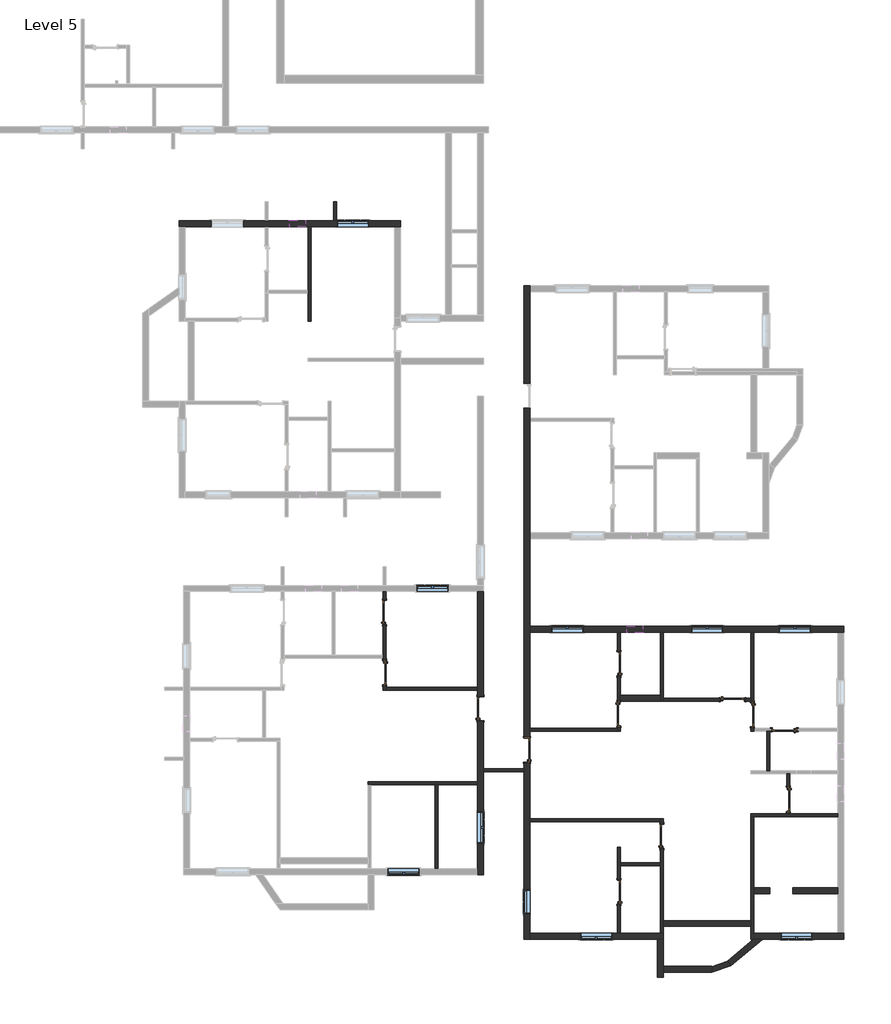
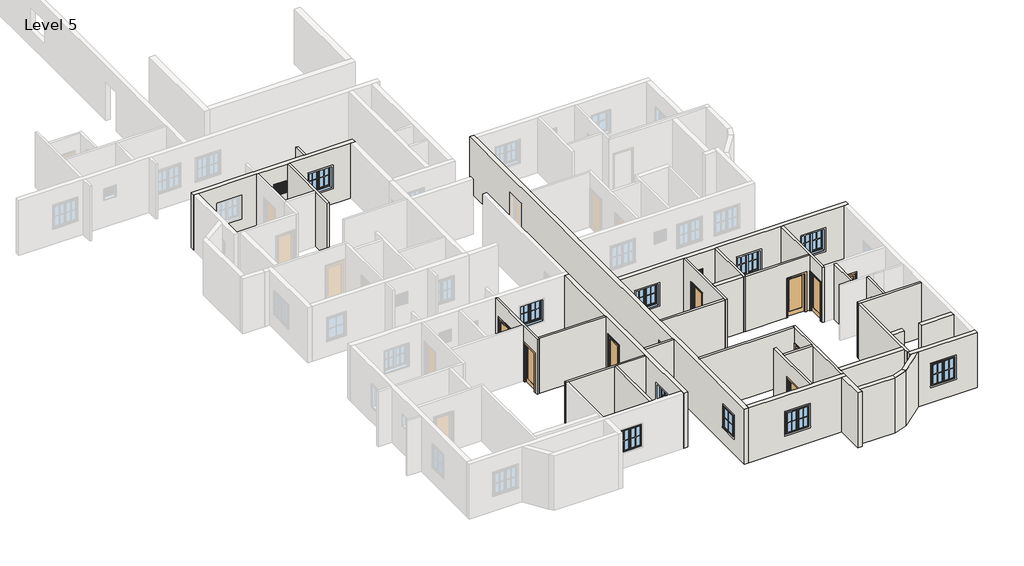
# One storey, part 2 of 7: 34 walls, 12 doors, 12 windows.
# Revit data of these elements (continued)
# Element 48 (IfcWindow, "Window-Casement-Double : 4' x 4'") (continued)
#   Materials on its faces: "Wood - Stained", "Glass", "Clad - White"
# Element 49 (IfcWindow, "Window-Casement-Double : 4' x 4'")
#   Mark = "112"
#   Window Inset = 0' - 0"
#   Interior Wall Closure = 0' - 2 1/4"
#   Frame Extension = 0' - 0 1/4"
#   Exterior Wall Closure = 0' - 1 1/4"
#   Interior Trim Visibility = yes
#   Exterior Trim Visibility = yes
#   Phase Created = New Construction
#   Materials on its faces: "Wood - Stained", "Glass", "Clad - White"
# Element 50 (IfcWindow, "Window-Casement-Double : 4' x 4'")
#   Mark = "113"
#   Window Inset = 0' - 0"
#   Interior Wall Closure = 0' - 2 1/4"
#   Frame Extension = 0' - 0 1/4"
#   Exterior Wall Closure = 0' - 1 1/4"
#   Interior Trim Visibility = yes
#   Exterior Trim Visibility = yes
#   Phase Created = New Construction
#   Materials on its faces: "Wood - Stained", "Glass", "Clad - White"
# Element 51 (IfcWindow, "Window-Casement-Double : 4' x 4'")
#   Mark = "114"
#   Window Inset = 0' - 0"
#   Interior Wall Closure = 0' - 2 1/4"
#   Frame Extension = 0' - 0 1/4"
#   Exterior Wall Closure = 0' - 1 1/4"
#   Interior Trim Visibility = yes
#   Exterior Trim Visibility = yes
#   Phase Created = New Construction
#   Materials on its faces: "Wood - Stained", "Glass", "Clad - White"
# Element 52 (IfcWindow, "Window-Casement-Double : 4' x 4'")
#   Mark = "115"
#   Window Inset = 0' - 0"
#   Interior Wall Closure = 0' - 2 1/4"
#   Frame Extension = 0' - 0 1/4"
#   Exterior Wall Closure = 0' - 1 1/4"
#   Interior Trim Visibility = yes
#   Exterior Trim Visibility = yes
#   Phase Created = New Construction
#   Materials on its faces: "Wood - Stained", "Glass", "Clad - White"
# Element 53 (IfcWindow, "Window-Casement-Double : 4' x 4'")
#   Mark = "116"
#   Window Inset = 0' - 0"
#   Interior Wall Closure = 0' - 2 1/4"
#   Frame Extension = 0' - 0 1/4"
#   Exterior Wall Closure = 0' - 1 1/4"
#   Interior Trim Visibility = yes
#   Exterior Trim Visibility = yes
#   Phase Created = New Construction
#   Materials on its faces: "Wood - Stained", "Glass", "Clad - White"
# Element 54 (IfcWindow, "Window-Casement-Double : 4' x 4'")
#   Mark = "117"
#   Window Inset = 0' - 0"
#   Interior Wall Closure = 0' - 2 1/4"
#   Frame Extension = 0' - 0 1/4"
#   Exterior Wall Closure = 0' - 1 1/4"
#   Interior Trim Visibility = yes
#   Exterior Trim Visibility = yes
#   Phase Created = New Construction
#   Materials on its faces: "Wood - Stained", "Glass", "Clad - White"
# Element 55 (IfcWindow, "Window-Casement-Double : 4' x 4'")
#   Mark = "119"
#   Window Inset = 0' - 0"
#   Interior Wall Closure = 0' - 2 1/4"
#   Frame Extension = 0' - 0 1/4"
#   Exterior Wall Closure = 0' - 1 1/4"
#   Interior Trim Visibility = yes
#   Exterior Trim Visibility = yes
#   Phase Created = New Construction
#   Materials on its faces: "Wood - Stained", "Glass", "Clad - White"
# Element 56 (IfcWindow, "Window-Casement-Double : 4' x 4'")
#   Mark = "126"
#   Window Inset = 0' - 0"
#   Interior Wall Closure = 0' - 2 1/4"
#   Frame Extension = 0' - 0 1/4"
#   Exterior Wall Closure = 0' - 1 1/4"
#   Interior Trim Visibility = yes
#   Exterior Trim Visibility = yes
#   Phase Created = New Construction
#   Materials on its faces: "Wood - Stained", "Glass", "Clad - White"
# Element 57 (IfcWindow, "Window-Louvers : 24\" x 24\"")
#   Mark = "73"
#   Blade Width = 1' - 10 1/2"
#   Phase Created = New Construction
#   Materials on its faces: "Birch"
# Element 58 (IfcWindow, "Window-Louvers : 24\" x 24\"")
#   Mark = "79"
#   Blade Width = 1' - 10 1/2"
#   Phase Created = New Construction
#   Materials on its faces: "Birch"
# Materials
#   "Cherry": class "Wood", colour RGB 226 177 128, transparency 0, Description = "Prunus Serotina", Cost = 0
#   "Aluminum": class "Metal", colour RGB 247 247 247, transparency 0, Description = "Aluminum 6061", Cost = 0
#   "Wood - Stained": class "Wood", colour RGB 224 178 126, transparency 0, Cost = 0
#   "Glass": class "Glass", colour RGB 0 128 192, transparency 0.75, Description = "Soda Lime Glass", Cost = 0
#   "Clad - White": class "Wood", colour RGB 242 242 238, transparency 0, Cost = 0
#   "Birch": class "Wood", colour RGB 224 178 126, transparency 0, Description = "Betula Alleghaniensis", Cost = 0
#   "Default Wall": colour RGB 128 128 128, transparency 0, Cost = 0
